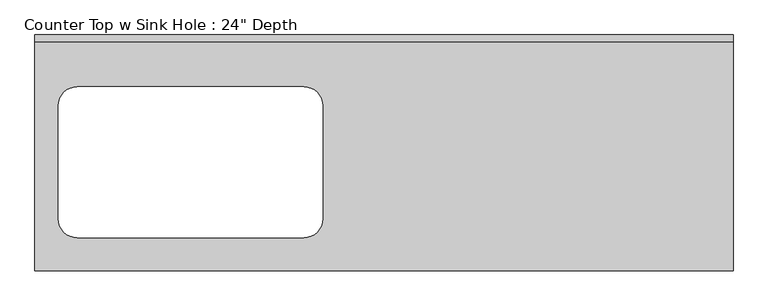
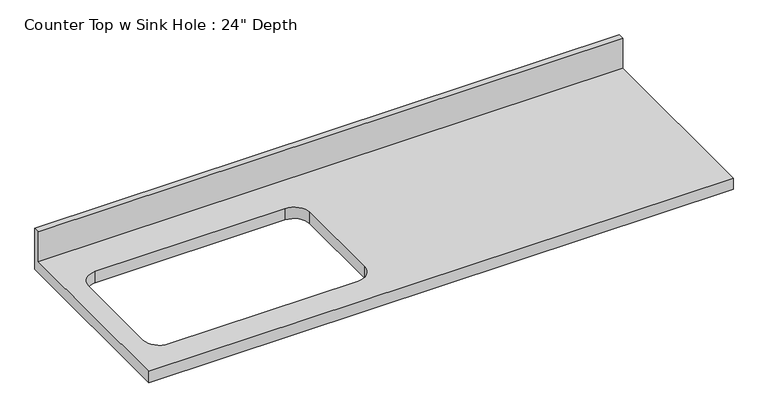
"""IFC4 building model written with IfcOpenShell, lengths in millimetres: furniture geometry."""

from ifc_helpers import new_model, si_unit, frame, origin, place, context, project, spatial, polyline, circle_curve, source, transform, mapped, element, save
from ifc_brep_helpers import plane_surface, revolved_surface, advanced_brep


def furniture_078eb3f3(model_context):
    return source(origin(), model_context, "Body", "AdvancedBrep", [
        advanced_brep(
        [(-1200.4622951, -635.0, 914.4), (678.8570745, -635.0, 914.4), (678.8570745, -19.05, 914.4), (-1200.4622951, -19.05, 914.4), (-1086.4429255, -139.7, 914.4), (-476.8429255, -139.7, 914.4), (-426.0429255, -190.5, 914.4), (-426.0429255, -495.3, 914.4), (-476.8429255, -546.1, 914.4), (-1086.4429255, -546.1, 914.4), (-1137.2429255, -495.3, 914.4), (-1137.2429255, -190.5, 914.4), (678.8570745, 0.0, 876.3), (678.8570745, -635.0, 876.3), (-1200.4622951, -635.0, 876.3), (-1200.4622951, 0.0, 876.3), (-476.8429255, -139.7, 876.3), (-1086.4429255, -139.7, 876.3), (-1137.2429255, -190.5, 876.3), (-1137.2429255, -495.3, 876.3), (-1086.4429255, -546.1, 876.3), (-476.8429255, -546.1, 876.3), (-426.0429255, -495.3, 876.3), (-426.0429255, -190.5, 876.3), (-1200.4622951, 0.0, 1016.0), (678.8570745, 0.0, 1016.0), (-1200.4622951, -19.05, 1016.0), (678.8570745, -19.05, 1016.0)],
        [
            (0, 1),
            (1, 2),
            (2, 3),
            (3, 0),
            (4, 5),
            (5, 6, circle_curve(frame((-476.8429255, -190.5, 914.4), z_axis=(0.0, 0.0, -1.0), x_axis=(1.0, 0.0, 0.0)), 50.8)),
            (6, 7),
            (7, 8, circle_curve(frame((-476.8429255, -495.3, 914.4), z_axis=(0.0, 0.0, -1.0), x_axis=(1.0, 0.0, 0.0)), 50.8)),
            (8, 9),
            (9, 10, circle_curve(frame((-1086.4429255, -495.3, 914.4), z_axis=(0.0, 0.0, -1.0), x_axis=(1.0, 0.0, 0.0)), 50.8)),
            (10, 11),
            (11, 4, circle_curve(frame((-1086.4429255, -190.5, 914.4), z_axis=(0.0, 0.0, -1.0), x_axis=(1.0, 0.0, 0.0)), 50.8)),
            (12, 13),
            (13, 14),
            (14, 15),
            (15, 12),
            (16, 17),
            (17, 18, circle_curve(frame((-1086.4429255, -190.5, 876.3), z_axis=(0.0, 0.0, 1.0), x_axis=(1.0, 0.0, 0.0)), 50.8)),
            (18, 19),
            (19, 20, circle_curve(frame((-1086.4429255, -495.3, 876.3), z_axis=(0.0, 0.0, 1.0), x_axis=(1.0, 0.0, 0.0)), 50.8)),
            (20, 21),
            (21, 22, circle_curve(frame((-476.8429255, -495.3, 876.3), z_axis=(0.0, 0.0, 1.0), x_axis=(1.0, 0.0, 0.0)), 50.8)),
            (22, 23),
            (23, 16, circle_curve(frame((-476.8429255, -190.5, 876.3), z_axis=(0.0, 0.0, 1.0), x_axis=(1.0, 0.0, 0.0)), 50.8)),
            (15, 24),
            (24, 25),
            (25, 12),
            (14, 0),
            (3, 26),
            (26, 24),
            (13, 1),
            (25, 27),
            (27, 2),
            (26, 27),
            (4, 17),
            (16, 5),
            (11, 18),
            (10, 19),
            (9, 20),
            (8, 21),
            (7, 22),
            (6, 23),
        ],
        [
            plane_surface(frame((-1200.4622951, 0.0, 914.4), z_axis=(0.0, 0.0, 1.0), x_axis=(-1.0, 0.0, 0.0))),
            plane_surface(frame((-1200.4622951, 0.0, 876.3), z_axis=(0.0, 0.0, -1.0), x_axis=(1.0, 0.0, 0.0))),
            plane_surface(frame((678.8570745, 0.0, 914.4), z_axis=(0.0, 1.0, 0.0), x_axis=(0.0, 0.0, -1.0))),
            plane_surface(frame((-1200.4622951, 0.0, 914.4), z_axis=(-1.0, 0.0, 0.0), x_axis=(0.0, 0.0, -1.0))),
            plane_surface(frame((-1200.4622951, -635.0, 914.4), z_axis=(0.0, -1.0, 0.0), x_axis=(0.0, 0.0, -1.0))),
            plane_surface(frame((678.8570745, -635.0, 914.4), z_axis=(1.0, 0.0, 0.0), x_axis=(0.0, 0.0, -1.0))),
            plane_surface(frame((-1200.4622951, 0.0, 1016.0), z_axis=(0.0, 0.0, 1.0), x_axis=(0.0, -1.0, 0.0))),
            plane_surface(frame((-1200.4622951, -19.05, 1016.0), z_axis=(0.0, -1.0, 0.0), x_axis=(0.0, 0.0, -1.0))),
            plane_surface(frame((-476.8429255, -139.7, 914.4), z_axis=(0.0, -1.0, 0.0), x_axis=(0.0, 0.0, -1.0))),
            revolved_surface(polyline([(-1035.6429255, -190.5, 914.4), (-1035.6429255, -190.5, 876.3)]), (-1086.4429255, -190.5, 876.3), (0.0, 0.0, 1.0)),
            plane_surface(frame((-1137.2429255, -190.5, 914.4), z_axis=(1.0, 0.0, 0.0), x_axis=(0.0, 0.0, -1.0))),
            revolved_surface(polyline([(-1035.6429255, -495.3, 914.4), (-1035.6429255, -495.3, 876.3)]), (-1086.4429255, -495.3, 876.3), (0.0, 0.0, 1.0)),
            plane_surface(frame((-1086.4429255, -546.1, 914.4), z_axis=(0.0, 1.0, 0.0), x_axis=(0.0, 0.0, -1.0))),
            revolved_surface(polyline([(-426.04292549999997, -495.3, 914.4), (-426.04292549999997, -495.3, 876.3)]), (-476.8429255, -495.3, 876.3), (0.0, 0.0, 1.0)),
            plane_surface(frame((-426.0429255, -495.3, 914.4), z_axis=(-1.0, 0.0, 0.0), x_axis=(0.0, 0.0, -1.0))),
            revolved_surface(polyline([(-426.04292549999997, -190.5, 914.4), (-426.04292549999997, -190.5, 876.3)]), (-476.8429255, -190.5, 876.3), (0.0, 0.0, 1.0)),
        ],
        [
            (0, [[1, 2, 3, 4], [5, 6, 7, 8, 9, 10, 11, 12]]),
            (1, [[13, 14, 15, 16], [17, 18, 19, 20, 21, 22, 23, 24]]),
            (2, [[-16, 25, 26, 27]]),
            (3, [[-15, 28, -4, 29, 30, -25]]),
            (4, [[-1, -28, -14, 31]]),
            (5, [[-13, -27, 32, 33, -2, -31]]),
            (6, [[-30, 34, -32, -26]]),
            (7, [[-34, -29, -3, -33]]),
            (8, [[35, -17, 36, -5]]),
            (9, [[-35, -12, 37, -18]]),
            (10, [[-37, -11, 38, -19]]),
            (11, [[-38, -10, 39, -20]]),
            (12, [[-39, -9, 40, -21]]),
            (13, [[-40, -8, 41, -22]]),
            (14, [[-41, -7, 42, -23]]),
            (15, [[-36, -24, -42, -6]]),
        ],
    ),
    ])


if __name__ == "__main__":
    model = new_model("IFC4")
    model_context = context("Model", 3, world=origin())
    ifc_project = project(units=[si_unit("LENGTHUNIT", "METRE", prefix="MILLI")], contexts=[model_context])
    site = spatial("IfcSite", under=ifc_project)
    building = spatial("IfcBuilding", under=site)
    placement = place(None, origin())
    furniture_shape = furniture_078eb3f3(model_context)
    element("IfcFurniture", 1, ObjectType="Counter Top w Sink Hole : 24\" Depth", at=placement, inside=building, context=model_context, shape_type="MappedRepresentation", body=[
        mapped(furniture_shape, transform((0.0, 0.0, 0.0), x_axis=(1.0, 0.0, 0.0), y_axis=(0.0, 1.0, 0.0), z_axis=(0.0, 0.0, 1.0))),
    ])
    save(model, "model.ifc")

# Revit data of these elements
# Type "Counter Top w Sink Hole : 24\" Depth"
#   Assembly Code = "C1030400"
#   Counter Thickness = 0.125 ft
#   Depth = 2.083333 ft
#   Height = 3 ft
#   Length [instance default] = 8 ft
#   Sink Location [instance default] = 2 ft
#   Sink Location To Wall [instance default] = 0.5 ft
#   Sink Opening Depth [instance default] = 1.25 ft
#   Sink Opening Width [instance default] = 2.25 ft
#   Counter Top Material = none
#   Default Elevation = 0
# Element 1 (IfcFurniture, "Counter Top w Sink Hole : 24\" Depth")
#   Length = 6.165746 ft
#   Sink Location = 1.374079 ft
#   Materials on its faces: "Counter Top"
# Materials
#   "Counter Top": class "Wood", colour RGB 226 177 128, transparency 0
